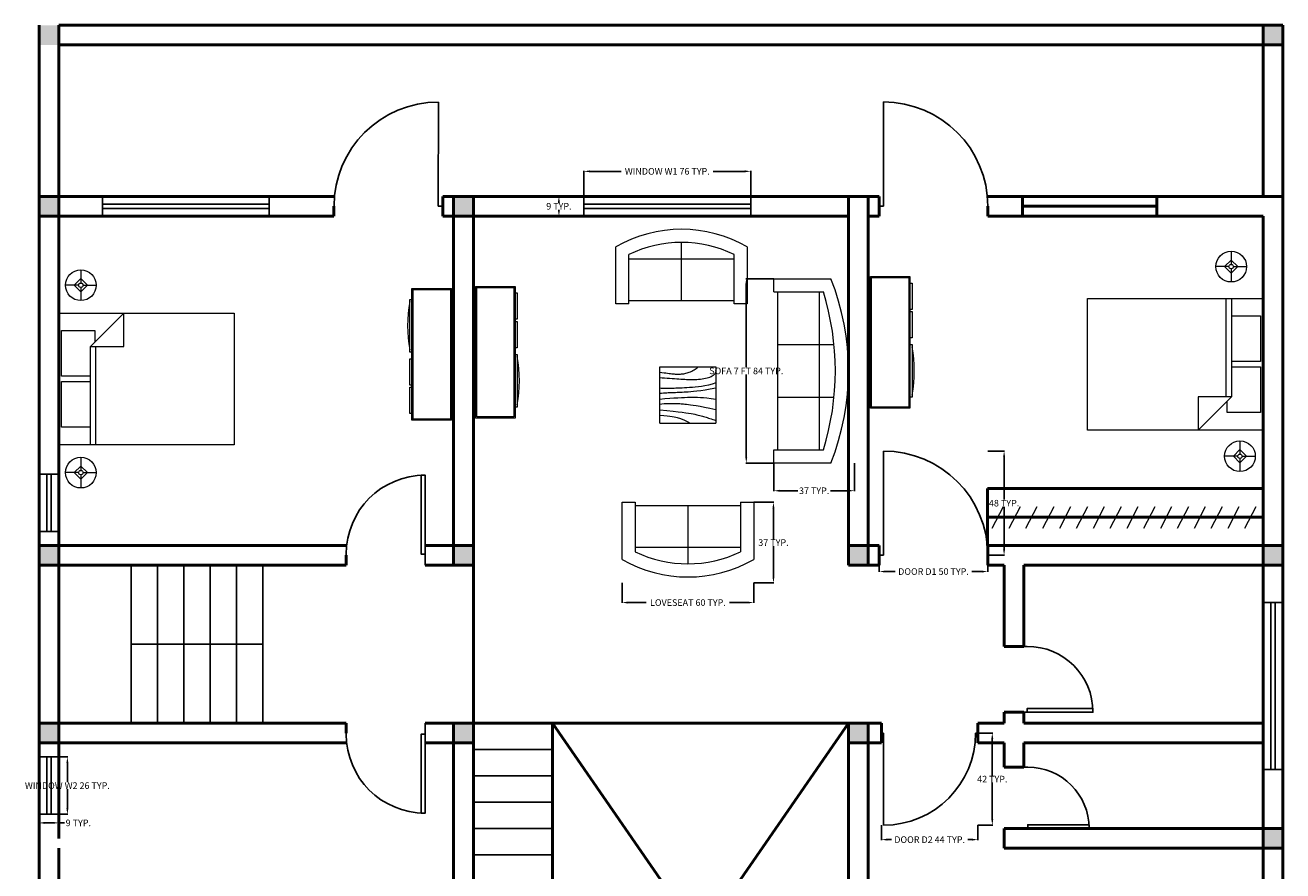
# Model space of a CAD drawing. Units: inches. Extents: x 13 to 1693, y -7 to 1519.
# Tile 9 of 10: x 1120 to 1693, y 350 to 735. Entities that reach past the tile are written whole.
import ezdxf

# ---------------------------------------------------------------- set-up
doc = ezdxf.new("R2010")
doc.units = ezdxf.units.IN
doc.header["$MEASUREMENT"] = 0
for name, color, linetype, lineweight in [('A-ANNO-DIMS', 2, 'Continuous', 18), ('A-DOOR', 4, 'Continuous', 25), ('A-FLOR-CASE', 5, 'Continuous', 18), ('A-FLOR-STRS', 2, 'Continuous', 25), ('A-FURN', 8, 'Continuous', 18), ('A-GLAZ', 4, 'Continuous', 25), ('A-WALL', 7, 'Continuous', 50), ('A-WALL-PATT', 8, 'Continuous', 13)]:
    doc.layers.add(name, color=color, linetype=linetype, lineweight=lineweight)
doc.styles.get("Standard").update_dxf_attribs({"font": 'arial.ttf'})
doc.dimstyles.get("Standard").update_dxf_attribs({"dimtxt": 3, "dimasz": 2.68, "dimexe": 0.18, "dimexo": 0.0625, "dimgap": 0.09, "dimtad": 0, "dimtih": 1, "dimtoh": 1, "dimdec": 0, "dimzin": 0, "dimdsep": 46, "dimlunit": 3, "dimtxsty": 'Standard', "dimcen": 0.09, "dimadec": 0, "dimazin": 0, "dimtfac": 1, "dimtdec": 0, "dimtofl": 0, "dimtmove": 0, "dimatfit": 3, "dimfxl": 1, "dimtolj": 1, "dimtzin": 0, "dimarcsym": 0})

# ---------------------------------------------------------------- blocks, each defined once
blk = doc.blocks.new('*U7')
for p, q in [((0, 0), (0, -5)), ((36, 0), (36, -5))]:
    blk.add_line(p, q)
blk.add_lwpolyline([(0, 0), (0, 36), (1.75, 36), (1.75, 0)], close=True)
blk.add_arc((0, 0), 36, 0, 90)
blk = doc.blocks.new('*U9')
for p, q in [((0, 0), (0, -6)), ((28, 0), (28, -6))]:
    blk.add_line(p, q)
blk.add_lwpolyline([(0, 0), (0, 28), (1.75, 28), (1.75, 0)], close=True)
blk.add_arc((0, 0), 28, 0, 90)
blk = doc.blocks.new('*U8')
for p, q in [((0, 0), (0, -6)), ((30, 0), (30, -6))]:
    blk.add_line(p, q)
blk.add_lwpolyline([(0, 0), (0, 30), (1.75, 30), (1.75, 0)], close=True)
blk.add_arc((0, 0), 30, 0, 90)
blk = doc.blocks.new('Sofa - Roundback Loveseat 5 ft.')
for p, q in [((0, -32.44198), (0, -5.99998)), ((-24, -33.99998), (-24, -11.46958)), ((-23.9998, -13.38178), (23.99986, -13.38178)), ((24.00004, -33.99998), (24.00004, -11.46958)), ((-24, -32.44198), (24.00004, -32.44198))]:
    blk.add_line(p, q)
for points in [[(-24, -33.99998), (-30, -33.99998), (-30, -7.99998)], [(30.00004, -7.99998), (30.00004, -33.99998), (24.00004, -33.99998)]]:
    blk.add_lwpolyline(points)
for centre, radius, start, end in [((0, -60.24998), 60.24998, 60.13715, 119.8628), ((0, -61.38438), 55.38444, 64.32083, 115.6792)]:
    blk.add_arc(centre, radius, start, end)
blk = doc.blocks.new('Bed - Queen')
for p, q in [((0, -80.00003), (0, 0)), ((0, 0), (59.99999, 0)), ((59.99999, 0), (59.99999, -80.00003)), ((7.99999, -1.2), (28.79998, -1.2)), ((7.99999, -14.4), (7.99999, -1.2)), ((28.79998, -1.2), (28.79998, -14.4)), ((31.19999, -1.2), (51.99999, -1.2)), ((31.19999, -14.4), (31.19999, -1.2)), ((51.99999, -1.2), (51.99999, -16.4)), ((0, -14.4), (44.8, -14.4)), ((44.8, -16.8), (0, -16.8)), ((59.99999, -29.6), (44.8, -14.4)), ((44.8, -14.4), (44.8, -29.6)), ((51.99999, -16.4), (46.79936, -16.4)), ((44.8, -29.6), (59.99999, -29.6)), ((59.99999, -80.00003), (0, -80.00003))]:
    blk.add_line(p, q)
blk = doc.blocks.new('Entertainment Center')
for p, q in [((-4, 0), (-5, -1)), ((4, 0), (-4, 0)), ((5, -1), (4, 0)), ((-17, -19), (-17, -1)), ((-17, -1), (43, -1)), ((-16.5, -18.5), (-16.5, -1.5)), ((-16.5, -1.5), (42.5, -1.5)), ((42.5, -1.5), (42.5, -18.5)), ((43, -1), (43, -19)), ((43, -19), (-17, -19)), ((42.5, -18.5), (-16.5, -18.5)), ((-12, -20), (-12, -19)), ((12, -20), (-12, -20)), ((12, -19), (12, -20)), ((15, -20), (15, -19)), ((27, -20), (15, -20)), ((27, -19), (27, -20)), ((28, -20), (28, -19)), ((40, -20), (28, -20)), ((40, -19), (40, -20))]:
    blk.add_line(p, q)
blk.add_arc((0, 40), 61, 259.6111, 280.3889)
blk = doc.blocks.new('Sofa - Roundback 7 ft.')
for p, q in [((-12.00002, -32.4421), (-12.00003, -6.5971)), ((11.99997, -32.4421), (11.99998, -6.5971)), ((-36.000027, -34), (-36.000027, -11.4696)), ((-35.999844, -13.3819), (35.9998, -13.3819)), ((35.99998, -34), (35.99998, -11.4696)), ((-36.000027, -32.4421), (35.99998, -32.4421))]:
    blk.add_line(p, q)
for points in [[(-36.000027, -34), (-42.000027, -34), (-42.000027, -8)], [(41.99998, -8), (41.99998, -34), (35.99998, -34)]]:
    blk.add_lwpolyline(points)
for centre, radius, start, end in [((0, -114.25), 114.25, 68.43141, 111.5686), ((-0.00001, -127.1968), 121.1968, 72.72033, 107.2797)]:
    blk.add_arc(centre, radius, start, end)
blk = doc.blocks.new('Table - Square Woodgrain 42 x 42 in.')
blk.add_line((0, -42), (42, -42))
for points in [[(0, -4), (1.704, -4.2172), (3.2358, -4.4188), (4.615, -4.604), (5.8615, -4.7721), (6.9951, -4.9224), (8.0357, -5.0541), (9.0031, -5.1667), (9.9171, -5.2594), (10.7951, -5.3316), (11.6445, -5.3836), (12.4702, -5.4157), (13.277, -5.4283), (14.0698, -5.4217), (14.8535, -5.3964), (15.6331, -5.3526), (16.4133, -5.2908), (17.1986, -5.2103), (17.9913, -5.1062), (18.793, -4.9727), (19.6056, -4.8038), (20.4307, -4.5937), (21.2701, -4.3365), (22.1256, -4.0262), (22.9989, -3.6571), (23.888, -3.2272), (24.7756, -2.7516), (25.6408, -2.2491), (26.4624, -1.7387), (27.2195, -1.2395), (27.891, -0.7703), (28.456, -0.3501), (28.8934, 0.002)], [(0, -42), (0, 0), (42, 0), (42, -42)], [(0, -8), (1.8203, -8.1001), (3.6741, -8.2149), (5.5411, -8.3408), (7.4011, -8.4741), (9.2339, -8.6112), (11.0193, -8.7484), (12.7371, -8.8821), (14.3671, -9.0086), (15.8954, -9.1246), (17.3337, -9.2278), (18.6997, -9.3159), (20.0116, -9.387), (21.2871, -9.4389), (22.5442, -9.4696), (23.8008, -9.477), (25.0749, -9.459), (26.3791, -9.4137), (27.7049, -9.3403), (29.0383, -9.2382), (30.3655, -9.1068), (31.6728, -8.9455), (32.9461, -8.7535), (34.1717, -8.5304), (35.3358, -8.2756), (36.4268, -7.9863), (37.443, -7.6521), (38.3849, -7.2603), (39.253, -6.7986), (40.048, -6.2542), (40.7705, -5.6147), (41.421, -4.8674), (42, -4)], [(42, -12), (39.1784, -12.8621), (36.4519, -13.5654), (33.8246, -14.1294), (31.3004, -14.5731), (28.8832, -14.9161), (26.577, -15.1775), (24.3858, -15.3768), (22.3136, -15.5332), (20.3622, -15.6632), (18.5254, -15.7718), (16.7947, -15.8612), (15.1618, -15.9338), (13.6183, -15.9916), (12.1558, -16.0369), (10.7659, -16.0718), (9.4403, -16.0987), (8.1703, -16.1191), (6.9461, -16.1325), (5.7577, -16.1377), (4.595, -16.1335), (3.4479, -16.1188), (2.3064, -16.0924), (1.1604, -16.0532), (0, -16)], [(42, -16), (37.6529, -16.7365), (33.8802, -17.329), (30.6179, -17.7961), (27.8015, -18.1561), (25.3668, -18.4275), (23.2497, -18.6288), (21.3859, -18.7785), (19.7111, -18.8949), (18.1693, -18.9939), (16.7375, -19.0795), (15.401, -19.1534), (14.1449, -19.217), (12.9544, -19.2717), (11.8148, -19.3191), (10.7113, -19.3606), (9.6291, -19.3976), (8.5534, -19.4323), (7.47, -19.4689), (6.3643, -19.5122), (5.222, -19.5672), (4.0288, -19.6386), (2.7703, -19.7313), (1.4321, -19.8501), (0, -20)], [(0, -24), (3.9243, -23.6805), (7.4766, -23.4138), (10.6891, -23.1954), (13.5943, -23.0205), (16.2247, -22.8847), (18.6125, -22.7832), (20.7903, -22.7116), (22.7903, -22.6651), (24.6563, -22.642), (26.4764, -22.6507), (28.35, -22.7024), (30.3766, -22.8084), (32.6555, -22.98), (35.2861, -23.2283), (38.3678, -23.5645), (42, -24)], [(42, -32), (37.392, -31.017), (33.4585, -30.2231), (30.1291, -29.5949), (27.3334, -29.109), (25.0009, -28.742), (23.0612, -28.4707), (21.4439, -28.2716), (20.0786, -28.1215), (18.8998, -28.0002), (17.8609, -27.9014), (16.9206, -27.8219), (16.0371, -27.7588), (15.1691, -27.709), (14.2748, -27.6693), (13.3128, -27.6368), (12.2415, -27.6083), (11.0295, -27.5824), (9.6867, -27.5643), (8.233, -27.5608), (6.6884, -27.5787), (5.0728, -27.6248), (3.4062, -27.7058), (1.7086, -27.8286), (0, -28)], [(0, -32), (5.4026, -32.5358), (9.9494, -33.019), (13.7424, -33.4553), (16.8834, -33.8505), (19.4743, -34.2106), (21.6171, -34.5413), (23.4136, -34.8486), (24.9657, -35.1382), (26.3614, -35.4156), (27.6332, -35.6841), (28.7995, -35.9467), (29.8788, -36.2064), (30.8897, -36.4661), (31.8507, -36.7288), (32.7802, -36.9973), (33.6968, -37.2747), (34.6175, -37.5635), (35.5531, -37.8651), (36.5128, -38.1805), (37.506, -38.5108), (38.5421, -38.8568), (39.6302, -39.2197), (40.7797, -39.6004), (42, -40)], [(0, -36), (3.0098, -36.2857), (5.5354, -36.5643), (7.6368, -36.8359), (9.374, -37.1009), (10.807, -37.3597), (11.9957, -37.6126), (13.0002, -37.8599), (13.8804, -38.102), (14.6874, -38.3393), (15.4365, -38.5729), (16.1338, -38.8041), (16.7858, -39.0341), (17.3987, -39.264), (17.9787, -39.4952), (18.5322, -39.7288), (19.0655, -39.9662), (19.5832, -40.2081), (20.0842, -40.4544), (20.5657, -40.7046), (21.0249, -40.9581), (21.459, -41.2144), (21.8653, -41.4731), (22.2409, -41.7335), (22.5831, -41.9951)]]:
    blk.add_lwpolyline(points)
blk = doc.blocks.new('Lamp - Table')
for p, q in [((0, 7), (0, 1)), ((-1, 0), (-7, 0)), ((0, 3), (-3, 0)), ((-3, 0), (0, -3)), ((3, 0), (0, 3)), ((0, -3), (3, 0)), ((1, 0), (7, 0)), ((0, -1), (0, -7))]:
    blk.add_line(p, q)
for radius in [7, 1]:
    blk.add_circle((0, 0), radius)
blk = doc.blocks.new('WIN-76')
for p, q in [((0, 9), (0, 0)), ((76.02, 9), (76.02, 0)), ((0, 5.5), (76.02, 5.5)), ((0, 3.5), (76.02, 3.5))]:
    blk.add_line(p, q)
blk = doc.blocks.new('WIN-26')
for p, q in [((9, 26.11), (0, 26.11)), ((3.5, 26.11), (3.5, 0)), ((5.5, 26.11), (5.5, 0)), ((9, 0), (0, 0))]:
    blk.add_line(p, q)
blk = doc.blocks.new('DOOR-42')
for p, q in [((0, 41.95), (1, 41.95)), ((1, 0), (1, 41.95)), ((43.95, 41.95), (42.95, 41.95))]:
    blk.add_line(p, q)
blk.add_arc((1, 41.95), 41.95, 270, 0)
blk = doc.blocks.new('DOOR-48')
for p, q in [((2, 0), (2, 47.5)), ((0, 0), (2, 0))]:
    blk.add_line(p, q)
blk.add_arc((2, 0), 47.5, 0, 90)
blk = doc.blocks.new('*D44')
at = {"layer": 'A-ANNO-DIMS', "color": 0, "lineweight": -2, "transparency": 16777216}
for p, q in [((1374.67, 657.21), (1374.67, 668.73)), ((1377.35, 668.55), (1391.72, 668.55)), ((1448.01, 668.55), (1433.63, 668.55)), ((1450.69, 657.21), (1450.69, 668.73))]:
    blk.add_line(p, q, dxfattribs=at)
at = {"layer": 'A-ANNO-DIMS', "color": 0, "transparency": 16777216}
for points in [[(1377.35, 669), (1377.35, 668.11), (1374.67, 668.55)], [(1448.01, 669), (1448.01, 668.11), (1450.69, 668.55)]]:
    blk.add_solid(points, dxfattribs=at)
at = {"layer": 'Defpoints', "color": 0, "transparency": 16777216}
for p in [(1374.67, 668.55), (1374.67, 657.15), (1450.69, 657.15)]:
    blk.add_point(p, dxfattribs=at)
at = {"layer": 'A-ANNO-DIMS', "color": 0, "transparency": 16777216, "insert": (1412.68, 668.55), "char_height": 3, "attachment_point": 5}
blk.add_mtext('\\A1;WINDOW W1 76 TYP.', dxfattribs=at)
blk = doc.blocks.new('*D45')
at = {"layer": 'A-ANNO-DIMS', "color": 0, "lineweight": -2, "transparency": 16777216}
for p, q in [((1374.6, 657.15), (1363.08, 657.15)), ((1363.26, 654.47), (1363.26, 654.27)), ((1374.6, 648.15), (1363.08, 648.15)), ((1363.26, 650.83), (1363.26, 651.03))]:
    blk.add_line(p, q, dxfattribs=at)
at = {"layer": 'A-ANNO-DIMS', "color": 0, "transparency": 16777216}
for points in [[(1362.82, 654.47), (1363.71, 654.47), (1363.26, 657.15)], [(1362.82, 650.83), (1363.71, 650.83), (1363.26, 648.15)]]:
    blk.add_solid(points, dxfattribs=at)
at = {"layer": 'Defpoints', "color": 0, "transparency": 16777216}
for p in [(1374.67, 657.15), (1363.26, 648.15), (1374.67, 648.15)]:
    blk.add_point(p, dxfattribs=at)
at = {"layer": 'A-ANNO-DIMS', "color": 0, "transparency": 16777216, "insert": (1363.26, 652.65), "char_height": 3, "attachment_point": 5}
blk.add_mtext('\\A1;9 TYP.', dxfattribs=at)
blk = doc.blocks.new('*D46')
at = {"layer": 'A-ANNO-DIMS', "color": 0, "lineweight": -2, "transparency": 16777216}
for p, q in [((1135.34, 401.76), (1139.38, 401.76)), ((1139.2, 399.08), (1139.2, 390.35)), ((1139.2, 378.33), (1139.2, 387.06)), ((1135.34, 375.65), (1139.38, 375.65))]:
    blk.add_line(p, q, dxfattribs=at)
at = {"layer": 'A-ANNO-DIMS', "color": 0, "transparency": 16777216}
for points in [[(1138.75, 399.08), (1139.64, 399.08), (1139.2, 401.76)], [(1138.75, 378.33), (1139.64, 378.33), (1139.2, 375.65)]]:
    blk.add_solid(points, dxfattribs=at)
at = {"layer": 'Defpoints', "color": 0, "transparency": 16777216}
for p in [(1135.28, 401.76), (1139.2, 401.76), (1135.28, 375.65)]:
    blk.add_point(p, dxfattribs=at)
at = {"layer": 'A-ANNO-DIMS', "color": 0, "transparency": 16777216, "insert": (1139.2, 388.71), "char_height": 3, "attachment_point": 5}
blk.add_mtext('\\A1;WINDOW W2 26 TYP.', dxfattribs=at)
blk = doc.blocks.new('*D47')
at = {"layer": 'A-ANNO-DIMS', "color": 0, "lineweight": -2, "transparency": 16777216}
for p, q in [((1126.28, 375.59), (1126.28, 371.55)), ((1135.28, 375.59), (1135.28, 371.55)), ((1128.96, 371.73), (1132.6, 371.73)), ((1135.28, 371.73), (1137.96, 371.73))]:
    blk.add_line(p, q, dxfattribs=at)
at = {"layer": 'A-ANNO-DIMS', "color": 0, "transparency": 16777216}
for points in [[(1128.96, 372.18), (1128.96, 371.29), (1126.28, 371.73)], [(1132.6, 372.18), (1132.6, 371.29), (1135.28, 371.73)]]:
    blk.add_solid(points, dxfattribs=at)
at = {"layer": 'Defpoints', "color": 0, "transparency": 16777216}
for p in [(1126.28, 375.65), (1135.28, 375.65), (1135.28, 371.73)]:
    blk.add_point(p, dxfattribs=at)
at = {"layer": 'A-ANNO-DIMS', "color": 0, "transparency": 16777216, "insert": (1144.19, 371.73), "char_height": 3, "attachment_point": 5}
blk.add_mtext('\\A1;9 TYP.', dxfattribs=at)
blk = doc.blocks.new('*D50')
at = {"layer": 'A-ANNO-DIMS', "color": 0, "lineweight": -2, "transparency": 16777216}
for p, q in [((1509.28, 493.59), (1509.28, 486.05)), ((1558.78, 493.59), (1558.78, 486.05)), ((1511.96, 486.23), (1516.58, 486.23)), ((1556.1, 486.23), (1551.48, 486.23))]:
    blk.add_line(p, q, dxfattribs=at)
at = {"layer": 'A-ANNO-DIMS', "color": 0, "transparency": 16777216}
for points in [[(1511.96, 486.67), (1511.96, 485.78), (1509.28, 486.23)], [(1556.1, 486.67), (1556.1, 485.78), (1558.78, 486.23)]]:
    blk.add_solid(points, dxfattribs=at)
at = {"layer": 'Defpoints', "color": 0, "transparency": 16777216}
for p in [(1509.28, 493.65), (1558.78, 493.65), (1558.78, 486.23)]:
    blk.add_point(p, dxfattribs=at)
at = {"layer": 'A-ANNO-DIMS', "color": 0, "transparency": 16777216, "insert": (1534.03, 486.23), "char_height": 3, "attachment_point": 5}
blk.add_mtext('\\A1;DOOR D1 50 TYP.', dxfattribs=at)
blk = doc.blocks.new('*D51')
at = {"layer": 'A-ANNO-DIMS', "color": 0, "lineweight": -2, "transparency": 16777216}
for p, q in [((1558.84, 541.15), (1566.39, 541.15)), ((1566.21, 538.47), (1566.21, 519.02)), ((1566.21, 496.33), (1566.21, 515.78)), ((1558.84, 493.65), (1566.39, 493.65))]:
    blk.add_line(p, q, dxfattribs=at)
at = {"layer": 'A-ANNO-DIMS', "color": 0, "transparency": 16777216}
for points in [[(1565.76, 538.47), (1566.65, 538.47), (1566.21, 541.15)], [(1565.76, 496.33), (1566.65, 496.33), (1566.21, 493.65)]]:
    blk.add_solid(points, dxfattribs=at)
at = {"layer": 'Defpoints', "color": 0, "transparency": 16777216}
for p in [(1558.78, 541.15), (1566.21, 541.15), (1558.78, 493.65)]:
    blk.add_point(p, dxfattribs=at)
at = {"layer": 'A-ANNO-DIMS', "color": 0, "transparency": 16777216, "insert": (1566.21, 517.4), "char_height": 3, "attachment_point": 5}
blk.add_mtext('\\A1;48 TYP.', dxfattribs=at)
blk = doc.blocks.new('*D52')
at = {"layer": 'A-ANNO-DIMS', "color": 0, "lineweight": -2, "transparency": 16777216}
for p, q in [((1510.28, 370.64), (1510.28, 363.92)), ((1554.23, 370.64), (1554.23, 363.92)), ((1512.96, 364.1), (1514.81, 364.1)), ((1551.55, 364.1), (1549.7, 364.1))]:
    blk.add_line(p, q, dxfattribs=at)
at = {"layer": 'A-ANNO-DIMS', "color": 0, "transparency": 16777216}
for points in [[(1512.96, 364.55), (1512.96, 363.66), (1510.28, 364.1)], [(1551.55, 364.55), (1551.55, 363.66), (1554.23, 364.1)]]:
    blk.add_solid(points, dxfattribs=at)
at = {"layer": 'Defpoints', "color": 0, "transparency": 16777216}
for p in [(1510.28, 370.7), (1554.23, 370.7), (1554.23, 364.1)]:
    blk.add_point(p, dxfattribs=at)
at = {"layer": 'A-ANNO-DIMS', "color": 0, "transparency": 16777216, "insert": (1532.26, 364.1), "char_height": 3, "attachment_point": 5}
blk.add_mtext('\\A1;DOOR D2 44 TYP.', dxfattribs=at)
blk = doc.blocks.new('*D53')
at = {"layer": 'A-ANNO-DIMS', "color": 0, "lineweight": -2, "transparency": 16777216}
for p, q in [((1554.3, 412.65), (1561.01, 412.65)), ((1560.83, 409.97), (1560.83, 393.27)), ((1560.83, 373.38), (1560.83, 390.08)), ((1554.3, 370.7), (1561.01, 370.7))]:
    blk.add_line(p, q, dxfattribs=at)
at = {"layer": 'A-ANNO-DIMS', "color": 0, "transparency": 16777216}
for points in [[(1560.38, 409.97), (1561.27, 409.97), (1560.83, 412.65)], [(1560.38, 373.38), (1561.27, 373.38), (1560.83, 370.7)]]:
    blk.add_solid(points, dxfattribs=at)
at = {"layer": 'Defpoints', "color": 0, "transparency": 16777216}
for p in [(1554.23, 412.65), (1560.83, 412.65), (1554.23, 370.7)]:
    blk.add_point(p, dxfattribs=at)
at = {"layer": 'A-ANNO-DIMS', "color": 0, "transparency": 16777216, "insert": (1560.83, 391.67), "char_height": 3, "attachment_point": 5}
blk.add_mtext('\\A1;42 TYP.', dxfattribs=at)
blk = doc.blocks.new('*D58')
at = {"layer": 'A-ANNO-DIMS', "color": 0, "lineweight": -2, "transparency": 16777216}
for p, q in [((1461.22, 619.65), (1448.5, 619.65)), ((1448.68, 616.97), (1448.68, 579.29)), ((1448.68, 538.33), (1448.68, 576.01)), ((1461.22, 535.65), (1448.5, 535.65))]:
    blk.add_line(p, q, dxfattribs=at)
at = {"layer": 'A-ANNO-DIMS', "color": 0, "transparency": 16777216}
for points in [[(1448.23, 616.97), (1449.13, 616.97), (1448.68, 619.65)], [(1448.23, 538.33), (1449.13, 538.33), (1448.68, 535.65)]]:
    blk.add_solid(points, dxfattribs=at)
at = {"layer": 'Defpoints', "color": 0, "transparency": 16777216}
for p in [(1461.28, 619.65), (1448.68, 535.65), (1461.28, 535.65)]:
    blk.add_point(p, dxfattribs=at)
at = {"layer": 'A-ANNO-DIMS', "color": 0, "transparency": 16777216, "insert": (1448.68, 577.65), "char_height": 3, "attachment_point": 5}
blk.add_mtext('\\A1;SOFA 7 FT 84 TYP.', dxfattribs=at)
blk = doc.blocks.new('*D59')
at = {"layer": 'A-ANNO-DIMS', "color": 0, "lineweight": -2, "transparency": 16777216}
for p, q in [((1461.28, 535.59), (1461.28, 522.87)), ((1497.95, 535.59), (1497.95, 522.87)), ((1463.96, 523.05), (1472.22, 523.05)), ((1495.27, 523.05), (1487, 523.05))]:
    blk.add_line(p, q, dxfattribs=at)
at = {"layer": 'A-ANNO-DIMS', "color": 0, "transparency": 16777216}
for points in [[(1463.96, 523.5), (1463.96, 522.6), (1461.28, 523.05)], [(1495.27, 523.5), (1495.27, 522.6), (1497.95, 523.05)]]:
    blk.add_solid(points, dxfattribs=at)
at = {"layer": 'Defpoints', "color": 0, "transparency": 16777216}
for p in [(1461.28, 535.65), (1497.95, 535.65), (1497.95, 523.05)]:
    blk.add_point(p, dxfattribs=at)
at = {"layer": 'A-ANNO-DIMS', "color": 0, "transparency": 16777216, "insert": (1479.61, 523.05), "char_height": 3, "attachment_point": 5}
blk.add_mtext('\\A1;37 TYP.', dxfattribs=at)
blk = doc.blocks.new('*D60')
at = {"layer": 'A-ANNO-DIMS', "color": 0, "lineweight": -2, "transparency": 16777216}
for p, q in [((1392.07, 481.04), (1392.07, 471.92)), ((1452.07, 481.04), (1452.07, 471.92)), ((1394.75, 472.1), (1403.1, 472.1)), ((1449.39, 472.1), (1441.04, 472.1))]:
    blk.add_line(p, q, dxfattribs=at)
at = {"layer": 'A-ANNO-DIMS', "color": 0, "transparency": 16777216}
for points in [[(1394.75, 472.55), (1394.75, 471.66), (1392.07, 472.1)], [(1449.39, 472.55), (1449.39, 471.66), (1452.07, 472.1)]]:
    blk.add_solid(points, dxfattribs=at)
at = {"layer": 'Defpoints', "color": 0, "transparency": 16777216}
for p in [(1392.07, 481.1), (1452.07, 481.1), (1392.07, 472.1)]:
    blk.add_point(p, dxfattribs=at)
at = {"layer": 'A-ANNO-DIMS', "color": 0, "transparency": 16777216, "insert": (1422.07, 472.1), "char_height": 3, "attachment_point": 5}
blk.add_mtext('\\A1;LOVESEAT 60 TYP.', dxfattribs=at)
blk = doc.blocks.new('*D61')
at = {"layer": 'A-ANNO-DIMS', "color": 0, "lineweight": -2, "transparency": 16777216}
for p, q in [((1452.13, 517.77), (1461.25, 517.77)), ((1461.07, 515.09), (1461.07, 501.06)), ((1461.07, 483.78), (1461.07, 497.82)), ((1452.13, 481.1), (1461.25, 481.1))]:
    blk.add_line(p, q, dxfattribs=at)
at = {"layer": 'A-ANNO-DIMS', "color": 0, "transparency": 16777216}
for points in [[(1460.62, 515.09), (1461.51, 515.09), (1461.07, 517.77)], [(1460.62, 483.78), (1461.51, 483.78), (1461.07, 481.1)]]:
    blk.add_solid(points, dxfattribs=at)
at = {"layer": 'Defpoints', "color": 0, "transparency": 16777216}
for p in [(1452.07, 517.77), (1452.07, 481.1), (1461.07, 481.1)]:
    blk.add_point(p, dxfattribs=at)
at = {"layer": 'A-ANNO-DIMS', "color": 0, "transparency": 16777216, "insert": (1461.07, 499.44), "char_height": 3, "attachment_point": 5}
blk.add_mtext('\\A1;37 TYP.', dxfattribs=at)

msp = doc.modelspace()

# ---------------------------------------------------------------- hatches: boundary and pattern name
at = {"layer": 'A-WALL-PATT'}
h = msp.add_hatch(color=256, dxfattribs=at)
h.dxf.hatch_style = 1
h.paths.add_polyline_path([(1135.28, 735.15), (1126.28, 735.15), (1126.28, 726.15), (1135.28, 726.15)])
h.paths.add_polyline_path([(1135.28, 657.15), (1126.28, 657.15), (1126.28, 648.15), (1135.28, 648.15)])
h.paths.add_polyline_path([(1135.28, 498.15), (1126.28, 498.15), (1126.28, 489.15), (1135.28, 489.15)])
h.paths.add_polyline_path([(1135.28, 417.15), (1126.28, 417.15), (1126.28, 408.15), (1135.28, 408.15)])
h.paths.add_polyline_path([(1135.28, 177.15), (1126.28, 177.15), (1126.28, 168.15), (1135.28, 168.15)])
h.paths.add_polyline_path([(1324.28, 177.15), (1315.28, 177.15), (1315.28, 168.15), (1324.28, 168.15)])
h.paths.add_polyline_path([(1324.28, 417.15), (1315.28, 417.15), (1315.28, 408.15), (1324.28, 408.15)])
h.paths.add_polyline_path([(1324.28, 498.15), (1315.28, 498.15), (1315.28, 489.15), (1324.28, 489.15)])
h.paths.add_polyline_path([(1324.28, 657.15), (1315.28, 657.15), (1315.28, 648.15), (1324.28, 648.15)])
h = msp.add_hatch(color=256, dxfattribs=at)
h.dxf.hatch_style = 1
h.paths.add_polyline_path([(1693.28, 735.15), (1684.28, 735.15), (1684.28, 726.15), (1693.28, 726.15)])
h.paths.add_polyline_path([(1504.28, 498.15), (1495.28, 498.15), (1495.28, 489.15), (1504.28, 489.15)])
h.paths.add_polyline_path([(1693.28, 498.15), (1684.28, 498.15), (1684.28, 489.15), (1693.28, 489.15)])
h.paths.add_polyline_path([(1693.28, 369.15), (1684.28, 369.15), (1684.28, 360.15), (1693.28, 360.15)])
h = msp.add_hatch(color=256, dxfattribs=at)
h.dxf.hatch_style = 1
h.paths.add_polyline_path([(1504.28, 417.15), (1495.28, 417.15), (1495.28, 408.15), (1504.28, 408.15)])

# ---------------------------------------------------------------- linework, layer by layer
at = {"layer": 'A-FLOR-CASE'}
for p, q in [((1565.8, 515.68), (1560.68, 505.81)), ((1573.48, 515.68), (1568.36, 505.81)), ((1581.16, 515.68), (1576.04, 505.81)), ((1588.83, 515.68), (1583.72, 505.81)), ((1596.51, 515.68), (1591.39, 505.81)), ((1604.19, 515.68), (1599.07, 505.81)), ((1611.87, 515.68), (1606.75, 505.81)), ((1619.54, 515.68), (1614.43, 505.81)), ((1627.22, 515.68), (1622.1, 505.81)), ((1634.9, 515.68), (1629.78, 505.81)), ((1642.58, 515.68), (1637.46, 505.81)), ((1650.25, 515.68), (1645.14, 505.81)), ((1657.93, 515.68), (1652.81, 505.81)), ((1665.61, 515.68), (1660.49, 505.81)), ((1673.29, 515.68), (1668.17, 505.81)), ((1680.96, 515.68), (1675.85, 505.81))]:
    msp.add_line(p, q, dxfattribs=at)
at = {"layer": 'A-FLOR-STRS'}
for p, q in [((1168.24, 489.15), (1168.24, 417.15)), ((1180.24, 489.15), (1180.24, 417.15)), ((1192.24, 489.15), (1192.24, 417.15)), ((1204.24, 489.15), (1204.24, 417.15)), ((1216.24, 489.15), (1216.24, 417.15)), ((1228.24, 489.15), (1228.24, 417.15)), ((1168.24, 453.15), (1228.24, 453.15)), ((1324.28, 405.15), (1360.28, 405.15)), ((1324.28, 393.15), (1360.28, 393.15)), ((1324.28, 381.15), (1360.28, 381.15)), ((1324.28, 369.15), (1360.28, 369.15)), ((1324.28, 357.15), (1360.28, 357.15))]:
    msp.add_line(p, q, dxfattribs=at)
at = {"layer": 'A-WALL'}
for p, q in [((1126.28, 168.15), (1126.28, 735.15)), ((1135.28, 364.65), (1135.28, 735.15)), ((1135.28, 735.15), (1684.28, 735.15)), ((1693.28, 168.15), (1693.28, 735.15)), ((1684.28, 726.15), (1135.28, 726.15)), ((1684.28, 657.15), (1684.28, 726.15)), ((1135.28, 657.15), (1126.28, 657.15)), ((1260.92, 657.15), (1126.28, 657.15)), ((1509.28, 657.15), (1310.28, 657.15)), ((1310.28, 657.15), (1310.28, 648.15)), ((1315.28, 657.15), (1315.28, 489.15)), ((1348.28, 657.15), (1315.28, 657.15)), ((1324.28, 657.15), (1324.28, 489.15)), ((1495.28, 498.15), (1495.28, 657.15)), ((1504.28, 498.15), (1504.28, 657.15)), ((1509.28, 648.15), (1509.28, 657.15)), ((1693.28, 657.15), (1558.57, 657.15)), ((1574.56, 657.15), (1574.56, 648.15)), ((1635.89, 648.15), (1635.89, 657.15)), ((1135.28, 648.15), (1126.28, 648.15)), ((1260.69, 648.15), (1126.28, 648.15)), ((1260.69, 648.15), (1260.69, 652.65)), ((1495.28, 648.15), (1310.28, 648.15)), ((1348.28, 648.15), (1315.28, 648.15)), ((1509.28, 648.15), (1504.28, 648.15)), ((1558.78, 648.15), (1558.78, 652.65)), ((1684.28, 648.15), (1558.78, 648.15)), ((1574.56, 652.65), (1635.89, 652.65)), ((1684.28, 498.15), (1684.28, 648.15)), ((1558.57, 498.15), (1558.57, 524.01)), ((1558.57, 524.01), (1684.28, 524.01)), ((1558.57, 511.08), (1684.28, 511.08)), ((1266.5, 498.15), (1126.28, 498.15)), ((1266.28, 493.65), (1266.28, 489.15)), ((1315.28, 498.15), (1302.28, 498.15)), ((1495.28, 489.15), (1495.28, 498.15)), ((1509.28, 498.15), (1495.28, 498.15)), ((1504.28, 489.15), (1504.28, 498.15)), ((1509.28, 489.15), (1509.28, 498.15)), ((1558.78, 498.15), (1558.57, 498.15)), ((1684.28, 498.15), (1558.78, 498.15)), ((1558.78, 489.15), (1558.78, 498.15)), ((1684.28, 489.15), (1684.28, 498.15)), ((1693.28, 498.15), (1684.28, 498.15)), ((1693.28, 489.15), (1693.28, 498.15)), ((1266.28, 489.15), (1126.28, 489.15)), ((1303.28, 489.15), (1302.28, 489.15)), ((1324.28, 489.15), (1303.28, 489.15)), ((1324.28, 489.15), (1324.28, 417.15)), ((1509.28, 489.15), (1495.28, 489.15)), ((1504.28, 489.15), (1509.28, 489.15)), ((1566.23, 489.15), (1558.78, 489.15)), ((1566.23, 489.15), (1566.23, 452.15)), ((1684.28, 489.15), (1575.23, 489.15)), ((1575.23, 489.15), (1575.23, 452.15)), ((1684.28, 369.15), (1684.28, 489.15)), ((1693.28, 489.15), (1684.28, 489.15)), ((1566.23, 452.15), (1575.23, 452.15)), ((1566.23, 422.15), (1566.23, 417.15)), ((1566.23, 417.15), (1566.23, 422.15)), ((1566.23, 422.15), (1575.23, 422.15)), ((1575.23, 422.15), (1575.23, 417.15)), ((1266.28, 417.15), (1126.28, 417.15)), ((1266.28, 412.65), (1266.28, 417.15)), ((1303.28, 417.15), (1302.28, 417.15)), ((1324.28, 417.15), (1303.28, 417.15)), ((1315.28, 417.15), (1315.28, 168.15)), ((1324.28, 417.15), (1324.28, 222.15)), ((1324.28, 417.15), (1360.28, 417.15)), ((1360.28, 417.15), (1360.28, 222.15)), ((1360.28, 417.15), (1495.28, 222.15)), ((1360.28, 222.15), (1495.28, 417.15)), ((1495.28, 213.15), (1495.28, 417.15)), ((1510.28, 417.15), (1495.28, 417.15)), ((1510.28, 408.15), (1510.28, 417.15)), ((1554.23, 408.15), (1554.23, 417.15)), ((1566.23, 417.15), (1554.23, 417.15)), ((1684.28, 417.15), (1575.23, 417.15)), ((1266.5, 408.15), (1126.28, 408.15)), ((1315.28, 408.15), (1302.28, 408.15)), ((1504.28, 213.15), (1504.28, 408.15)), ((1510.28, 408.15), (1504.28, 408.15)), ((1566.23, 408.15), (1554.23, 408.15)), ((1566.23, 408.15), (1566.23, 397.15)), ((1566.23, 408.15), (1566.23, 406.15)), ((1684.28, 408.15), (1575.23, 408.15)), ((1575.23, 406.15), (1575.23, 408.15)), ((1575.23, 408.15), (1575.23, 397.15)), ((1566.23, 397.15), (1575.23, 397.15)), ((1575.23, 369.15), (1566.23, 369.15)), ((1566.23, 369.15), (1566.23, 360.15)), ((1684.28, 369.15), (1575.23, 369.15)), ((1135.28, 168.15), (1135.28, 360.15)), ((1684.28, 360.15), (1566.23, 360.15)), ((1684.28, 168.15), (1684.28, 360.15))]:
    msp.add_line(p, q, dxfattribs=at)
for points in [[(1504.28, 735.15), (1495.28, 735.15)], [(1495.28, 726.15), (1504.28, 726.15)]]:
    msp.add_lwpolyline(points, dxfattribs=at)
for points in [[(1693.28, 735.15), (1684.28, 735.15), (1684.28, 726.15), (1693.28, 726.15)], [(1126.28, 489.15), (1135.28, 489.15), (1135.28, 498.15), (1126.28, 498.15)], [(1315.28, 489.15), (1324.28, 489.15), (1324.28, 498.15), (1315.28, 498.15)], [(1126.28, 408.15), (1135.28, 408.15), (1135.28, 417.15), (1126.28, 417.15)], [(1315.28, 408.15), (1324.28, 408.15), (1324.28, 417.15), (1315.28, 417.15)], [(1360.28, 222.15), (1495.28, 222.15), (1495.28, 417.15), (1360.28, 417.15)], [(1495.28, 417.15), (1504.28, 417.15), (1504.28, 408.15), (1495.28, 408.15)], [(1684.28, 369.15), (1693.28, 369.15), (1693.28, 360.15), (1684.28, 360.15)]]:
    msp.add_lwpolyline(points, close=True, dxfattribs=at)

# ---------------------------------------------------------------- block references
at = {"layer": 'A-DOOR', "extrusion": (0, 0, -1), "zscale": -1, "rotation": 0.0629583221345953}
msp.add_blockref('DOOR-48', (-1310.26, 652.62), dxfattribs=at)
at = {"layer": 'A-DOOR'}
for name, p in [('DOOR-48', (1509.28, 652.65)), ('DOOR-48', (1509.28, 493.65)), ('DOOR-42', (1510.28, 370.7))]:
    msp.add_blockref(name, p, dxfattribs=at)
at = {"layer": 'A-DOOR', "xscale": -1}
msp.add_blockref('*U7', (1302.28, 494.15), dxfattribs=at)
at = {"layer": 'A-DOOR', "xscale": -1, "rotation": 270}
for name, p in [('*U8', (1576.73, 422.15)), ('*U9', (1576.98, 369.15))]:
    msp.add_blockref(name, p, dxfattribs=at)
at = {"layer": 'A-DOOR', "rotation": 180}
msp.add_blockref('*U7', (1302.28, 412.15), dxfattribs=at)
at = {"layer": 'A-FURN'}
for name, p in [('Sofa - Roundback Loveseat 5 ft.', (1419.16, 642.15)), ('Lamp - Table', (1669.73, 625.15)), ('Lamp - Table', (1145.33, 616.68)), ('Lamp - Table', (1673.73, 538.77)), ('Lamp - Table', (1145.33, 531.3))]:
    msp.add_blockref(name, p, dxfattribs=at)
for name, p, rotation in [('Sofa - Roundback 7 ft.', (1495.28, 577.65), 270), ('Entertainment Center', (1504.28, 577.65), 90), ('Entertainment Center', (1315.28, 598.21), 270), ('Entertainment Center', (1324.28, 573.15), 90), ('Bed - Queen', (1684.28, 610.67), 270), ('Bed - Queen', (1135.28, 544), 90), ('Sofa - Roundback Loveseat 5 ft.', (1422.07, 483.77), 180)]:
    msp.add_blockref(name, p, dxfattribs=dict(at, rotation=rotation))
at = {"layer": 'A-FURN', "xscale": 0.6108650724074032, "yscale": 0.6108650724074032, "zscale": 0.6108650724074032}
msp.add_blockref('Table - Square Woodgrain 42 x 42 in.', (1409.2, 579.5), dxfattribs=at)
at = {"layer": 'A-GLAZ'}
for name, p, rotation in [('WIN-76', (1231.22, 657.15), 180), ('WIN-76', (1450.69, 657.15), 180), ('WIN-26', (1135.28, 530.65), 180), ('WIN-76', (1684.28, 472.13), 270.0000000000003)]:
    msp.add_blockref(name, p, dxfattribs=dict(at, rotation=rotation))
msp.add_blockref('WIN-26', (1126.28, 375.65), dxfattribs=at)

# ---------------------------------------------------------------- dimensions: what is measured, and where the dimension line sits
at = {"layer": 'A-ANNO-DIMS'}
for base, p1, p2, angle, text, picture, middle in [((1374.67, 668.55), (1450.69, 657.15), (1374.67, 657.15), 180, 'WINDOW W1 <> TYP.', '*D44', (1412.68, 668.55)), ((1363.26, 648.15), (1374.67, 657.15), (1374.67, 648.15), 270, '<> TYP.', '*D45', (1363.26, 652.65)), ((1448.68, 535.65), (1461.28, 619.65), (1461.28, 535.65), 270, 'SOFA 7 FT <> TYP.', '*D58', (1448.68, 577.65)), ((1566.20525146, 541.15086621), (1558.78025146, 493.65086621), (1558.78025146, 541.15086621), 90, '<> TYP.', '*D51', (1566.20525146, 517.40086621)), ((1461.07, 481.1), (1452.07, 517.77), (1452.07, 481.1), 270, '<> TYP.', '*D61', (1461.07, 499.44)), ((1392.07, 472.1), (1452.07, 481.1), (1392.07, 481.1), 180, 'LOVESEAT <> TYP.', '*D60', (1422.07, 472.1)), ((1560.83, 412.65), (1554.23, 370.7), (1554.23, 412.65), 90, '<> TYP.', '*D53', (1560.83, 391.67)), ((1139.2, 401.76), (1135.28, 375.65), (1135.28, 401.76), 90, 'WINDOW W2 <> TYP.', '*D46', (1139.2, 388.71))]:
    dim = msp.add_linear_dim(base=base, p1=p1, p2=p2, angle=angle, text=text, dimstyle='Standard', override={"dimdec": 0, "dimlfac": 1, "dimrnd": 0, "dimzin": 0, "dimdsep": 46, "dimlunit": 2}, dxfattribs=at)
    dim.commit()
    dim.dimension.update_dxf_attribs({"geometry": picture, "text_midpoint": middle})
for base, p1, p2, text, picture, middle in [((1497.95, 523.05), (1461.28, 535.65), (1497.95, 535.65), '<> TYP.', '*D59', (1479.61, 523.05)), ((1558.78025146, 486.22586621), (1509.28025146, 493.65086621), (1558.78025146, 493.65086621), 'DOOR D1 <> TYP.', '*D50', (1534.03025146, 486.22586621)), ((1135.28, 371.73), (1126.28, 375.65), (1135.28, 375.65), '<> TYP.', '*D47', (1144.19, 371.73)), ((1554.23, 364.1), (1510.28, 370.7), (1554.23, 370.7), 'DOOR D2 <> TYP.', '*D52', (1532.26, 364.1))]:
    dim = msp.add_linear_dim(base=base, p1=p1, p2=p2, text=text, dimstyle='Standard', override={"dimdec": 0, "dimlfac": 1, "dimrnd": 0, "dimzin": 0, "dimdsep": 46, "dimlunit": 2}, dxfattribs=at)
    dim.commit()
    dim.dimension.update_dxf_attribs({"geometry": picture, "text_midpoint": middle})

doc.saveas('drawing.dxf')
